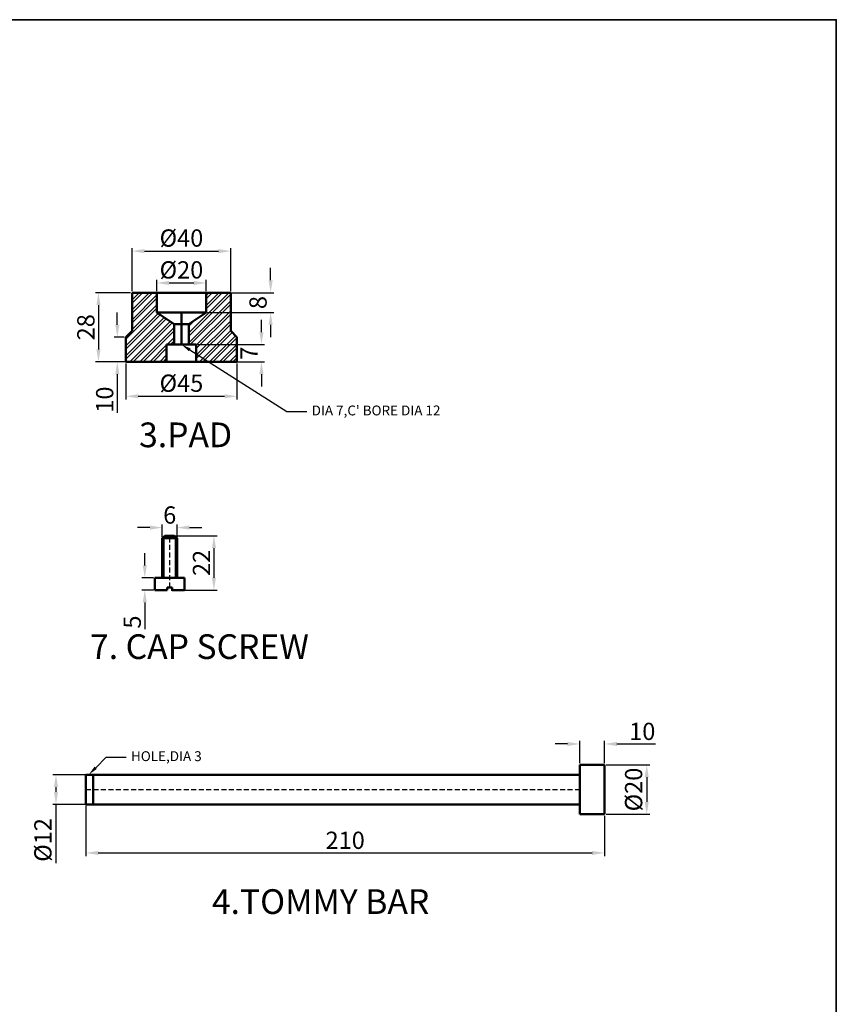
# Model space of a CAD drawing. Units: millimetres. Extents: x 210 to 1120, y -242 to 418.
# Tile 4 of 4: x 789 to 1120, y 20 to 418. Entities that reach past the tile are written whole.
import ezdxf
from ezdxf import colors
from ezdxf.entities.mleader import LeaderData, LeaderLine
from ezdxf.math import Vec2, Vec3

# ---------------------------------------------------------------- set-up
doc = ezdxf.new("R2010")
doc.units = ezdxf.units.MM
doc.header["$LTSCALE"] = 0.4
doc.linetypes.add('DASHED', pattern=[19.05, 12.7, -6.35])
for name, color, linetype, lineweight in [('M-DIMS', 2, 'Continuous', 25), ('M-HATC', 8, 'Continuous', 18), ('M-HIDN', 4, 'DASHED', 25), ('M-OUTL', 7, 'Continuous', 50), ('M-TEXT', 3, 'Continuous', 25), ('M-TTLB', 7, 'Continuous', 35)]:
    doc.layers.add(name, color=color, linetype=linetype, lineweight=lineweight)
doc.styles.get("Standard").update_dxf_attribs({"font": 'arial.ttf'})
doc.dimstyles.new('ISO-25', dxfattribs={"dimtxt": 7, "dimasz": 5, "dimexe": 1.25, "dimexo": 0.625, "dimtad": 1, "dimtxsty": 'Standard', "dimcen": 2.5, "dimadec": 0, "dimazin": 0, "dimtfac": 1, "dimtofl": 0, "dimtmove": 0, "dimatfit": 3, "dimfxl": 1, "dimarcsym": 0})

# ---------------------------------------------------------------- blocks, each defined once
blk = doc.blocks.new('*D26')
at = {"layer": 'Defpoints', "color": 0, "ltscale": 0.4, "transparency": 16777216}
for p in [(834.35, 307.81), (820.76, 279.81), (834.35, 279.81)]:
    blk.add_point(p, dxfattribs=at)
at = {"layer": 'M-DIMS', "color": 0, "lineweight": -2, "ltscale": 0.4, "transparency": 16777216}
for p, q in [((833.72, 307.81), (819.51, 307.81)), ((820.76, 302.81), (820.76, 284.81)), ((833.72, 279.81), (819.51, 279.81))]:
    blk.add_line(p, q, dxfattribs=at)
at = {"layer": 'M-DIMS', "color": 0, "ltscale": 0.4, "transparency": 16777216}
for points in [[(819.93, 302.81), (821.59, 302.81), (820.76, 307.81)], [(819.93, 284.81), (821.59, 284.81), (820.76, 279.81)]]:
    blk.add_solid(points, dxfattribs=at)
at = {"layer": 'M-DIMS', "color": 0, "ltscale": 0.4, "transparency": 16777216, "insert": (816.56, 293.81), "char_height": 7, "attachment_point": 5, "rotation": 90}
blk.add_mtext('28', dxfattribs=at)
blk = doc.blocks.new('*D27')
at = {"layer": 'Defpoints', "color": 0, "ltscale": 0.4, "transparency": 16777216}
for p in [(831.85, 289.81), (828.38, 279.81), (831.85, 279.81)]:
    blk.add_point(p, dxfattribs=at)
at = {"layer": 'M-DIMS', "color": 0, "lineweight": -2, "ltscale": 0.4, "transparency": 16777216}
for p, q in [((828.38, 294.81), (828.38, 299.81)), ((831.22, 289.81), (827.13, 289.81)), ((831.22, 279.81), (827.13, 279.81)), ((828.38, 274.81), (828.38, 259.21))]:
    blk.add_line(p, q, dxfattribs=at)
at = {"layer": 'M-DIMS', "color": 0, "ltscale": 0.4, "transparency": 16777216}
for points in [[(827.55, 294.81), (829.21, 294.81), (828.38, 289.81)], [(827.55, 274.81), (829.21, 274.81), (828.38, 279.81)]]:
    blk.add_solid(points, dxfattribs=at)
at = {"layer": 'M-DIMS', "color": 0, "ltscale": 0.4, "transparency": 16777216, "insert": (824.18, 264.51), "char_height": 7, "attachment_point": 5, "rotation": 90}
blk.add_mtext('10', dxfattribs=at)
blk = doc.blocks.new('*D28')
at = {"layer": 'Defpoints', "color": 0, "ltscale": 0.4, "transparency": 16777216}
for p in [(864.35, 307.81), (864.35, 299.81), (890.47, 299.81)]:
    blk.add_point(p, dxfattribs=at)
at = {"layer": 'M-DIMS', "color": 0, "lineweight": -2, "ltscale": 0.4, "transparency": 16777216}
for p, q in [((890.47, 312.81), (890.47, 317.81)), ((864.97, 307.81), (891.72, 307.81)), ((864.97, 299.81), (891.72, 299.81)), ((890.47, 294.81), (890.47, 289.81))]:
    blk.add_line(p, q, dxfattribs=at)
at = {"layer": 'M-DIMS', "color": 0, "ltscale": 0.4, "transparency": 16777216}
for points in [[(889.64, 312.81), (891.31, 312.81), (890.47, 307.81)], [(889.64, 294.81), (891.31, 294.81), (890.47, 299.81)]]:
    blk.add_solid(points, dxfattribs=at)
at = {"layer": 'M-DIMS', "color": 0, "ltscale": 0.4, "transparency": 16777216, "insert": (886.27, 303.81), "char_height": 7, "attachment_point": 5, "rotation": 90}
blk.add_mtext('8', dxfattribs=at)
blk = doc.blocks.new('*D29')
at = {"layer": 'Defpoints', "color": 0, "ltscale": 0.4, "transparency": 16777216}
for p in [(860.35, 286.81), (860.35, 279.81), (886.77, 279.81)]:
    blk.add_point(p, dxfattribs=at)
at = {"layer": 'M-DIMS', "color": 0, "lineweight": -2, "ltscale": 0.4, "transparency": 16777216}
for p, q in [((886.77, 291.81), (886.77, 296.81)), ((860.97, 286.81), (888.02, 286.81)), ((860.97, 279.81), (888.02, 279.81)), ((886.77, 274.81), (886.77, 269.81))]:
    blk.add_line(p, q, dxfattribs=at)
at = {"layer": 'M-DIMS', "color": 0, "ltscale": 0.4, "transparency": 16777216}
for points in [[(885.93, 291.81), (887.6, 291.81), (886.77, 286.81)], [(885.93, 274.81), (887.6, 274.81), (886.77, 279.81)]]:
    blk.add_solid(points, dxfattribs=at)
at = {"layer": 'M-DIMS', "color": 0, "ltscale": 0.4, "transparency": 16777216, "insert": (882.64, 283.31), "char_height": 7, "attachment_point": 5, "rotation": 90}
blk.add_mtext('7', dxfattribs=at)
blk = doc.blocks.new('*D30')
at = {"layer": 'Defpoints', "color": 0, "ltscale": 0.4, "transparency": 16777216}
for p in [(831.85, 279.81), (876.85, 279.81), (876.85, 265.86)]:
    blk.add_point(p, dxfattribs=at)
at = {"layer": 'M-DIMS', "color": 0, "lineweight": -2, "ltscale": 0.4, "transparency": 16777216}
for p, q in [((831.85, 279.18), (831.85, 264.61)), ((876.85, 279.18), (876.85, 264.61)), ((836.85, 265.86), (871.85, 265.86))]:
    blk.add_line(p, q, dxfattribs=at)
at = {"layer": 'M-DIMS', "color": 0, "ltscale": 0.4, "transparency": 16777216}
for points in [[(836.85, 266.69), (836.85, 265.03), (831.85, 265.86)], [(871.85, 266.69), (871.85, 265.03), (876.85, 265.86)]]:
    blk.add_solid(points, dxfattribs=at)
at = {"layer": 'M-DIMS', "color": 0, "ltscale": 0.4, "transparency": 16777216, "insert": (854.35, 270.25), "char_height": 7, "attachment_point": 5}
blk.add_mtext('%%C45', dxfattribs=at)
blk = doc.blocks.new('*D31')
at = {"layer": 'Defpoints', "color": 0, "ltscale": 0.4, "transparency": 16777216}
for p in [(864.35, 311.74), (844.35, 307.81), (864.35, 307.81)]:
    blk.add_point(p, dxfattribs=at)
at = {"layer": 'M-DIMS', "color": 0, "lineweight": -2, "ltscale": 0.4, "transparency": 16777216}
for p, q in [((844.35, 308.43), (844.35, 312.99)), ((849.35, 311.74), (859.35, 311.74)), ((864.35, 308.43), (864.35, 312.99))]:
    blk.add_line(p, q, dxfattribs=at)
at = {"layer": 'M-DIMS', "color": 0, "ltscale": 0.4, "transparency": 16777216}
for points in [[(849.35, 312.57), (849.35, 310.91), (844.35, 311.74)], [(859.35, 312.57), (859.35, 310.91), (864.35, 311.74)]]:
    blk.add_solid(points, dxfattribs=at)
at = {"layer": 'M-DIMS', "color": 0, "ltscale": 0.4, "transparency": 16777216, "insert": (854.35, 316.13), "char_height": 7, "attachment_point": 5}
blk.add_mtext('%%C20', dxfattribs=at)
blk = doc.blocks.new('*D32')
at = {"layer": 'Defpoints', "color": 0, "ltscale": 0.4, "transparency": 16777216}
for p in [(874.35, 324.64), (834.35, 307.81), (874.35, 307.81)]:
    blk.add_point(p, dxfattribs=at)
at = {"layer": 'M-DIMS', "color": 0, "lineweight": -2, "ltscale": 0.4, "transparency": 16777216}
for p, q in [((834.35, 308.43), (834.35, 325.89)), ((839.35, 324.64), (869.35, 324.64)), ((874.35, 308.43), (874.35, 325.89))]:
    blk.add_line(p, q, dxfattribs=at)
at = {"layer": 'M-DIMS', "color": 0, "ltscale": 0.4, "transparency": 16777216}
for points in [[(839.35, 325.47), (839.35, 323.8), (834.35, 324.64)], [(869.35, 325.47), (869.35, 323.8), (874.35, 324.64)]]:
    blk.add_solid(points, dxfattribs=at)
at = {"layer": 'M-DIMS', "color": 0, "ltscale": 0.4, "transparency": 16777216, "insert": (854.35, 329.03), "char_height": 7, "attachment_point": 5}
blk.add_mtext('%%C40', dxfattribs=at)
blk = doc.blocks.new('*D34')
at = {"layer": 'Defpoints', "color": 0, "ltscale": 0.4, "transparency": 16777216}
for p in [(849.6, 209.38), (849.6, 187.38), (867.51, 187.38)]:
    blk.add_point(p, dxfattribs=at)
at = {"layer": 'M-DIMS', "color": 0, "lineweight": -2, "ltscale": 0.4, "transparency": 16777216}
for p, q in [((850.23, 209.38), (868.76, 209.38)), ((867.51, 204.38), (867.51, 192.38)), ((850.23, 187.38), (868.76, 187.38))]:
    blk.add_line(p, q, dxfattribs=at)
at = {"layer": 'M-DIMS', "color": 0, "ltscale": 0.4, "transparency": 16777216}
for points in [[(866.68, 204.38), (868.35, 204.38), (867.51, 209.38)], [(866.68, 192.38), (868.35, 192.38), (867.51, 187.38)]]:
    blk.add_solid(points, dxfattribs=at)
at = {"layer": 'M-DIMS', "color": 0, "ltscale": 0.4, "transparency": 16777216, "insert": (863.38, 198.38), "char_height": 7, "attachment_point": 5, "rotation": 90}
blk.add_mtext('22', dxfattribs=at)
blk = doc.blocks.new('*D35')
at = {"layer": 'Defpoints', "color": 0, "ltscale": 0.4, "transparency": 16777216}
for p in [(852.6, 212.68), (846.6, 208.38), (852.6, 208.38)]:
    blk.add_point(p, dxfattribs=at)
at = {"layer": 'M-DIMS', "color": 0, "lineweight": -2, "ltscale": 0.4, "transparency": 16777216}
for p, q in [((841.6, 212.68), (836.6, 212.68)), ((846.6, 209), (846.6, 213.93)), ((852.6, 209), (852.6, 213.93)), ((857.6, 212.68), (862.6, 212.68))]:
    blk.add_line(p, q, dxfattribs=at)
at = {"layer": 'M-DIMS', "color": 0, "ltscale": 0.4, "transparency": 16777216}
for points in [[(841.6, 213.51), (841.6, 211.85), (846.6, 212.68)], [(857.6, 213.51), (857.6, 211.85), (852.6, 212.68)]]:
    blk.add_solid(points, dxfattribs=at)
at = {"layer": 'M-DIMS', "color": 0, "ltscale": 0.4, "transparency": 16777216, "insert": (849.6, 216.88), "char_height": 7, "attachment_point": 5}
blk.add_mtext('6', dxfattribs=at)
blk = doc.blocks.new('*D36')
at = {"layer": 'Defpoints', "color": 0, "ltscale": 0.4, "transparency": 16777216}
for p in [(843.6, 192.38), (839.51, 187.38), (843.6, 187.38)]:
    blk.add_point(p, dxfattribs=at)
at = {"layer": 'M-DIMS', "color": 0, "lineweight": -2, "ltscale": 0.4, "transparency": 16777216}
for p, q in [((839.51, 197.38), (839.51, 202.38)), ((842.98, 192.38), (838.26, 192.38)), ((842.98, 187.38), (838.26, 187.38)), ((839.51, 182.38), (839.51, 171.49))]:
    blk.add_line(p, q, dxfattribs=at)
at = {"layer": 'M-DIMS', "color": 0, "ltscale": 0.4, "transparency": 16777216}
for points in [[(838.68, 197.38), (840.35, 197.38), (839.51, 192.38)], [(838.68, 182.38), (840.35, 182.38), (839.51, 187.38)]]:
    blk.add_solid(points, dxfattribs=at)
at = {"layer": 'M-DIMS', "color": 0, "ltscale": 0.4, "transparency": 16777216, "insert": (835.33, 174.43), "char_height": 7, "attachment_point": 5, "rotation": 90}
blk.add_mtext('5', dxfattribs=at)
blk = doc.blocks.new('*D37')
at = {"layer": 'Defpoints', "color": 0, "ltscale": 0.4, "transparency": 16777216}
for p in [(839.45, 112.62), (803.55, 100.62), (839.45, 100.62)]:
    blk.add_point(p, dxfattribs=at)
at = {"layer": 'M-DIMS', "color": 0, "lineweight": -2, "ltscale": 0.4, "transparency": 16777216}
for p, q in [((838.83, 112.62), (802.3, 112.62)), ((803.55, 107.62), (803.55, 105.62)), ((838.83, 100.62), (802.3, 100.62)), ((803.55, 100.62), (803.55, 76.79))]:
    blk.add_line(p, q, dxfattribs=at)
at = {"layer": 'M-DIMS', "color": 0, "ltscale": 0.4, "transparency": 16777216}
for points in [[(802.72, 107.62), (804.39, 107.62), (803.55, 112.62)], [(802.72, 105.62), (804.39, 105.62), (803.55, 100.62)]]:
    blk.add_solid(points, dxfattribs=at)
at = {"layer": 'M-DIMS', "color": 0, "ltscale": 0.4, "transparency": 16777216, "insert": (799.16, 86.21), "char_height": 7, "attachment_point": 5, "rotation": 90}
blk.add_mtext('%%C12', dxfattribs=at)
blk = doc.blocks.new('*D38')
at = {"layer": 'Defpoints', "color": 0, "ltscale": 0.4, "transparency": 16777216}
for p in [(1025.66, 116.62), (1025.66, 96.62), (1042.76, 96.62)]:
    blk.add_point(p, dxfattribs=at)
at = {"layer": 'M-DIMS', "color": 0, "lineweight": -2, "ltscale": 0.4, "transparency": 16777216}
for p, q in [((1026.28, 116.62), (1044.01, 116.62)), ((1042.76, 111.62), (1042.76, 101.62)), ((1026.28, 96.62), (1044.01, 96.62))]:
    blk.add_line(p, q, dxfattribs=at)
at = {"layer": 'M-DIMS', "color": 0, "ltscale": 0.4, "transparency": 16777216}
for points in [[(1041.93, 111.62), (1043.59, 111.62), (1042.76, 116.62)], [(1041.93, 101.62), (1043.59, 101.62), (1042.76, 96.62)]]:
    blk.add_solid(points, dxfattribs=at)
at = {"layer": 'M-DIMS', "color": 0, "ltscale": 0.4, "transparency": 16777216, "insert": (1038.36, 106.62), "char_height": 7, "attachment_point": 5, "rotation": 90}
blk.add_mtext('%%C20', dxfattribs=at)
blk = doc.blocks.new('*D39')
at = {"layer": 'Defpoints', "color": 0, "ltscale": 0.4, "transparency": 16777216}
for p in [(1025.66, 125.07), (1015.66, 116.62), (1025.66, 116.62)]:
    blk.add_point(p, dxfattribs=at)
at = {"layer": 'M-DIMS', "color": 0, "lineweight": -2, "ltscale": 0.4, "transparency": 16777216}
for p, q in [((1010.66, 125.07), (1005.66, 125.07)), ((1015.66, 117.24), (1015.66, 126.32)), ((1025.66, 117.24), (1025.66, 126.32)), ((1030.66, 125.07), (1046.25, 125.07))]:
    blk.add_line(p, q, dxfattribs=at)
at = {"layer": 'M-DIMS', "color": 0, "ltscale": 0.4, "transparency": 16777216}
for points in [[(1010.66, 125.9), (1010.66, 124.23), (1015.66, 125.07)], [(1030.66, 125.9), (1030.66, 124.23), (1025.66, 125.07)]]:
    blk.add_solid(points, dxfattribs=at)
at = {"layer": 'M-DIMS', "color": 0, "ltscale": 0.4, "transparency": 16777216, "insert": (1040.95, 129.26), "char_height": 7, "attachment_point": 5}
blk.add_mtext('10', dxfattribs=at)
blk = doc.blocks.new('*D40')
at = {"layer": 'Defpoints', "color": 0, "ltscale": 0.4, "transparency": 16777216}
for p in [(815.66, 100.62), (1025.66, 96.62), (1025.66, 80.95)]:
    blk.add_point(p, dxfattribs=at)
at = {"layer": 'M-DIMS', "color": 0, "lineweight": -2, "ltscale": 0.4, "transparency": 16777216}
for p, q in [((815.66, 99.99), (815.66, 79.7)), ((1025.66, 95.99), (1025.66, 79.7)), ((820.66, 80.95), (1020.66, 80.95))]:
    blk.add_line(p, q, dxfattribs=at)
at = {"layer": 'M-DIMS', "color": 0, "ltscale": 0.4, "transparency": 16777216}
for points in [[(820.66, 81.79), (820.66, 80.12), (815.66, 80.95)], [(1020.66, 81.79), (1020.66, 80.12), (1025.66, 80.95)]]:
    blk.add_solid(points, dxfattribs=at)
at = {"layer": 'M-DIMS', "color": 0, "ltscale": 0.4, "transparency": 16777216, "insert": (920.66, 85.15), "char_height": 7, "attachment_point": 5}
blk.add_mtext('210', dxfattribs=at)

msp = doc.modelspace()

# ---------------------------------------------------------------- hatches: boundary and pattern name
at = {"layer": 'M-HATC', "ltscale": 0.4}
h = msp.add_hatch(dxfattribs=at)
h.set_pattern_fill('ANSI32', color=256, scale=0.3)
h.paths.add_polyline_path([(851.348, 295.08), (844.348, 299.8085), (844.348, 307.8085), (834.348, 307.8085), (834.348, 292.3085), (831.848, 289.8085), (831.848, 279.8085), (848.348, 279.8085), (848.348, 286.8085), (851.348, 286.8085)])
h.paths.add_polyline_path([(874.348, 307.8085), (864.348, 307.8085), (864.348, 299.8085), (857.348, 295.08), (857.348, 286.8085), (860.348, 286.8085), (860.348, 279.8085), (876.848, 279.8085), (876.848, 289.8085), (874.348, 292.3085)])

# ---------------------------------------------------------------- linework, layer by layer
at = {"layer": 'M-HIDN', "ltscale": 0.4}
for p, q in [((849.601, 188.3799), (849.601, 209.3799)), ((815.6565, 106.6163), (1015.6565, 106.6163))]:
    msp.add_line(p, q, dxfattribs=at)
at = {"layer": 'M-OUTL', "ltscale": 0.4}
for p, q in [((854.348, 307.8085), (834.348, 307.8085)), ((834.348, 307.8085), (834.348, 292.3085)), ((844.348, 299.8085), (844.348, 307.8085)), ((854.348, 307.8085), (874.348, 307.8085)), ((864.348, 307.8085), (864.348, 299.8085)), ((874.348, 307.8085), (874.348, 292.3085)), ((864.348, 299.8085), (844.348, 299.8085)), ((851.348, 295.08), (844.348, 299.8085)), ((854.348, 286.8085), (854.348, 299.8085)), ((857.348, 295.08), (864.348, 299.8085)), ((851.348, 286.8085), (851.348, 295.08)), ((851.348, 295.08), (857.348, 295.08)), ((857.348, 286.8085), (857.348, 295.08)), ((831.848, 289.8085), (834.348, 292.3085)), ((876.848, 289.8085), (874.348, 292.3085)), ((831.848, 279.8085), (831.848, 289.8085)), ((876.848, 279.8085), (876.848, 289.8085)), ((860.348, 286.8085), (848.348, 286.8085)), ((848.348, 286.8085), (848.348, 279.8085)), ((860.348, 279.8085), (860.348, 286.8085)), ((831.848, 279.8085), (876.848, 279.8085)), ((846.601, 208.3799), (847.601, 209.3799)), ((846.601, 208.3799), (846.601, 192.3799)), ((846.601, 208.3799), (852.601, 208.3799)), ((847.101, 208.3799), (847.101, 192.3799)), ((847.601, 209.3799), (851.601, 209.3799)), ((852.601, 208.3799), (851.601, 209.3799)), ((852.101, 208.3799), (852.101, 192.3799)), ((852.601, 208.3799), (852.601, 192.3799)), ((855.601, 192.3799), (843.601, 192.3799)), ((843.601, 192.3799), (843.601, 187.3799)), ((855.601, 187.3799), (855.601, 192.3799)), ((848.601, 187.3799), (848.601, 188.3799)), ((848.601, 188.3799), (850.601, 188.3799)), ((850.601, 188.3799), (850.601, 187.3799)), ((843.601, 187.3799), (848.601, 187.3799)), ((850.601, 187.3799), (855.601, 187.3799)), ((1015.6565, 116.6163), (1025.6565, 116.6163)), ((1015.6565, 96.6163), (1015.6565, 116.6163)), ((1025.6565, 116.6163), (1025.6565, 96.6163)), ((815.6565, 112.6163), (1015.6565, 112.6163)), ((815.6565, 100.6163), (815.6565, 112.6163)), ((818.6565, 100.6163), (818.6565, 112.6163)), ((815.6565, 100.6163), (1015.6565, 100.6163)), ((1025.6565, 96.6163), (1015.6565, 96.6163))]:
    msp.add_line(p, q, dxfattribs=at)
at = {"layer": 'M-TTLB', "ltscale": 0.4}
msp.add_lwpolyline([(210.1659, 418.3486), (1119.5264, 418.3486), (1119.5264, -242.3444), (210.1659, -242.3444)], close=True, dxfattribs=at)

# ---------------------------------------------------------------- texts
at = {"layer": 'M-TEXT', "attachment_point": 1}
for s, width, insert, char_height in [('\\pxqc;{\\H0.66667x;3.PAD} ', 102.831898, (804.6384, 255.2405), 15), ('\\pxqc;7. CAP SCREW', 157.820403, (782.7472, 169.4836), 10), ('\\pxqc;{\\H0.66667x;4.TOMMY BAR} ', 159.738723, (830.8318, 66.2441), 15)]:
    msp.add_mtext_dynamic_manual_height_columns(s, width=width, gutter_width=12.5, heights=[0], dxfattribs=dict(at, insert=insert, char_height=char_height))

# ---------------------------------------------------------------- dimensions: what is measured, and where the dimension line sits
at = {"layer": 'M-DIMS', "ltscale": 0.4}
for base, p1, p2, picture, middle in [((874.348, 324.6382), (834.348, 307.8085), (874.348, 307.8085), '*D32', (854.348, 329.033)), ((864.348, 311.7398), (844.348, 307.8085), (864.348, 307.8085), '*D31', (854.348, 316.1346)), ((876.848, 265.8585), (831.848, 279.8085), (876.848, 279.8085), '*D30', (854.348, 270.2532))]:
    dim = msp.add_linear_dim(base=base, p1=p1, p2=p2, text='%%C<>', dimstyle='ISO-25', override={"dimclrd": 0, "dimclre": 0, "dimclrt": 0}, dxfattribs=at)
    dim.commit()
    dim.dimension.update_dxf_attribs({"geometry": picture, "text_midpoint": middle})
for base, p1, p2, picture, middle in [((890.4725, 299.8085), (864.348, 307.8085), (864.348, 299.8085), '*D28', (886.2735, 303.8085)), ((820.7595, 279.8085), (834.348, 307.8085), (834.348, 279.8085), '*D26', (816.5605, 293.8085)), ((828.3809, 279.8085), (831.848, 289.8085), (831.848, 279.8085), '*D27', (824.1819, 264.5112)), ((886.7678, 279.8085), (860.348, 286.8085), (860.348, 279.8085), '*D29', (882.6428, 283.3085)), ((867.5147, 187.3799), (849.601, 209.3799), (849.601, 187.3799), '*D34', (863.3754, 198.3799)), ((839.5144, 187.3799), (843.601, 192.3799), (843.601, 187.3799), '*D36', (835.3297, 174.4343))]:
    dim = msp.add_linear_dim(base=base, p1=p1, p2=p2, angle=90, dimstyle='ISO-25', override={"dimclrd": 0, "dimclre": 0, "dimclrt": 0}, dxfattribs=at)
    dim.commit()
    dim.dimension.update_dxf_attribs({"geometry": picture, "text_midpoint": middle})
for base, p1, p2, picture, middle in [((852.601, 212.6788), (846.601, 208.3799), (852.601, 208.3799), '*D35', (849.601, 216.8778)), ((1025.6565, 125.0652), (1015.6565, 116.6163), (1025.6565, 116.6163), '*D39', (1040.9537, 129.2642)), ((1025.6565, 80.9517), (815.6565, 100.6163), (1025.6565, 96.6163), '*D40', (920.6565, 85.1507))]:
    dim = msp.add_linear_dim(base=base, p1=p1, p2=p2, dimstyle='ISO-25', override={"dimclrd": 0, "dimclre": 0, "dimclrt": 0}, dxfattribs=at)
    dim.commit()
    dim.dimension.update_dxf_attribs({"geometry": picture, "text_midpoint": middle})
for base, p1, p2, picture, middle in [((1042.7593, 96.6163), (1025.6565, 116.6163), (1025.6565, 96.6163), '*D38', (1038.3645, 106.6163)), ((803.5529, 100.6163), (839.4505, 112.6163), (839.4505, 100.6163), '*D37', (799.1581, 86.2055))]:
    dim = msp.add_linear_dim(base=base, p1=p1, p2=p2, angle=90, text='%%C<>', dimstyle='ISO-25', override={"dimclrd": 0, "dimclre": 0, "dimclrt": 0}, dxfattribs=at)
    dim.commit()
    dim.dimension.update_dxf_attribs({"geometry": picture, "text_midpoint": middle})

# ---------------------------------------------------------------- leaders
at = {"layer": 'M-TEXT', "ltscale": 0.4}
ml = msp.add_multileader_mtext('Standard', dxfattribs=at)
ml.set_content("DIA 7,C' BORE DIA 12", color=256)
ml.set_leader_properties()
ml.build(insert=Vec2(0, 0))
ctx = ml.context
ctx.base_point, ctx.plane_origin = Vec3(905.0909, 259.7205), Vec3(860.348, 279.8085)
notes = []
notes.append((ctx, [(0, (1, 1, 0), (897.0909, 259.7205), (1, 0), 8, [(0, [(854.348, 286.8085)], 0, [])])]))
ctx.mtext.insert, ctx.mtext.flow_direction = Vec3(907.0909, 262.1161), 5
ml = msp.add_multileader_mtext('Standard', dxfattribs=at)
ml.set_content('HOLE,DIA 3', color=256)
ml.set_leader_properties()
ml.build(insert=Vec2(0, 0))
ctx = ml.context
ctx.base_point, ctx.plane_origin = Vec3(831.9209, 119.7286), Vec3(816.8086, 112.6163)
notes.append((ctx, [(0, (1, 1, 0), (823.9209, 119.7286), (1, 0), 8, [(0, [(816.8086, 112.6163)], 0, [])])]))
ctx.mtext.insert, ctx.mtext.flow_direction = Vec3(833.9209, 122.1242), 5
for ctx, leaders in notes:
    for number, flags, end, landing, length, lines in leaders:
        leader = LeaderData()
        leader.index, (leader.has_last_leader_line, leader.has_dogleg_vector, leader.attachment_direction) = number, flags
        leader.last_leader_point, leader.dogleg_vector, leader.dogleg_length = Vec3(end), Vec3(landing), length
        for number, points, colour, breaks in lines:
            line = LeaderLine()
            line.index, line.vertices, line.color, line.breaks = number, Vec3.list(points), colors.encode_raw_color(colour), breaks
            leader.lines.append(line)
        ctx.leaders.append(leader)

doc.saveas('drawing.dxf')
